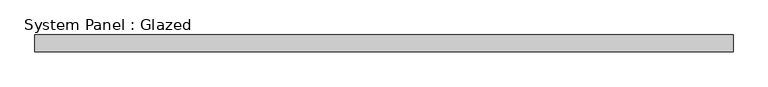
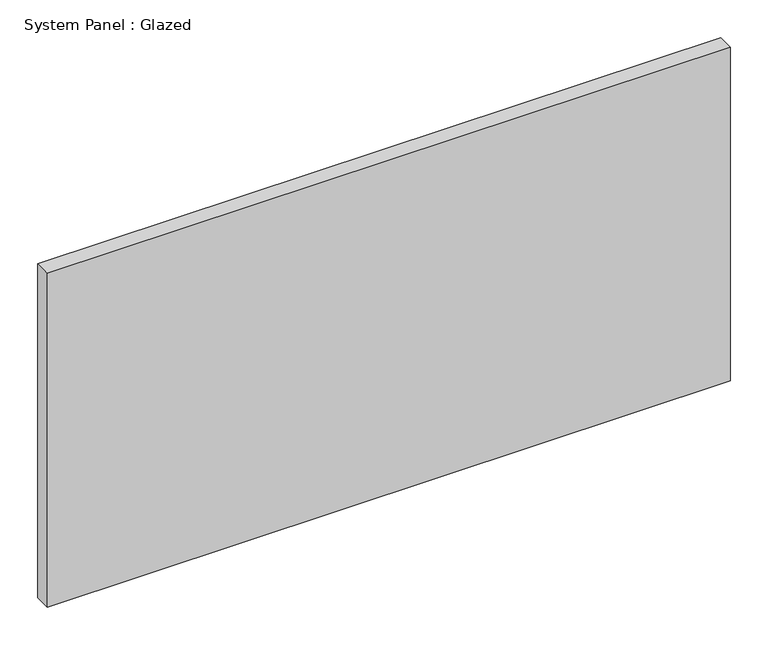
"""IFC4 building model written with IfcOpenShell, lengths in millimetres: plate geometry, System Panel : Glazed."""

from ifc_helpers import new_model, si_unit, origin, origin_with_axes, place, context, project, spatial, polyline, outline, extrude, source, transform, mapped, element, save


def system_panel_glazed_3447b65c(model_context):
    return source(origin(), model_context, "Body", "SweptSolid", [
        extrude(outline(polyline([(523.875, 19.05), (-523.875, 19.05), (-523.875, 44.45), (523.875, 44.45), (523.875, 19.05)])), origin_with_axes(), (0.0, 0.0, 1.0), 540.9706626),
    ])


if __name__ == "__main__":
    model = new_model("IFC4")
    model_context = context("Model", 3, world=origin())
    ifc_project = project(units=[si_unit("LENGTHUNIT", "METRE", prefix="MILLI")], contexts=[model_context])
    site = spatial("IfcSite", under=ifc_project)
    building = spatial("IfcBuilding", under=site)
    placement = place(None, origin())
    system_panel_glazed_shape = system_panel_glazed_3447b65c(model_context)
    element("IfcPlate", 1, ObjectType="System Panel : Glazed", at=placement, inside=building, context=model_context, shape_type="MappedRepresentation", body=[
        mapped(system_panel_glazed_shape, transform((0.0, 0.0, 0.0), x_axis=(1.0, 0.0, 0.0), y_axis=(0.0, 1.0, 0.0), z_axis=(0.0, 0.0, 1.0))),
    ])
    save(model, "model.ifc")

# Revit data of these elements
# Type "System Panel : Glazed"
#   Construction Type Id = "GSP4R"
#   Analytic Construction = "1/8 in Pilkington single glazing"
#   Visual Light Transmittance = 0.9
#   Solar Heat Gain Coefficient = 0.86
#   Heat Transfer Coefficient (U) = 1.18115 BTU/(h·ft²·°F)
#   Define Thermal Properties by = 1
# Element 1 (IfcPlate, "System Panel : Glazed")
#   Materials on its faces: "Glass"
# Materials
#   "Glass": class "Glass", colour RGB 0 128 192, transparency 0.75, Description = "Soda Lime Glass", Cost = 0
